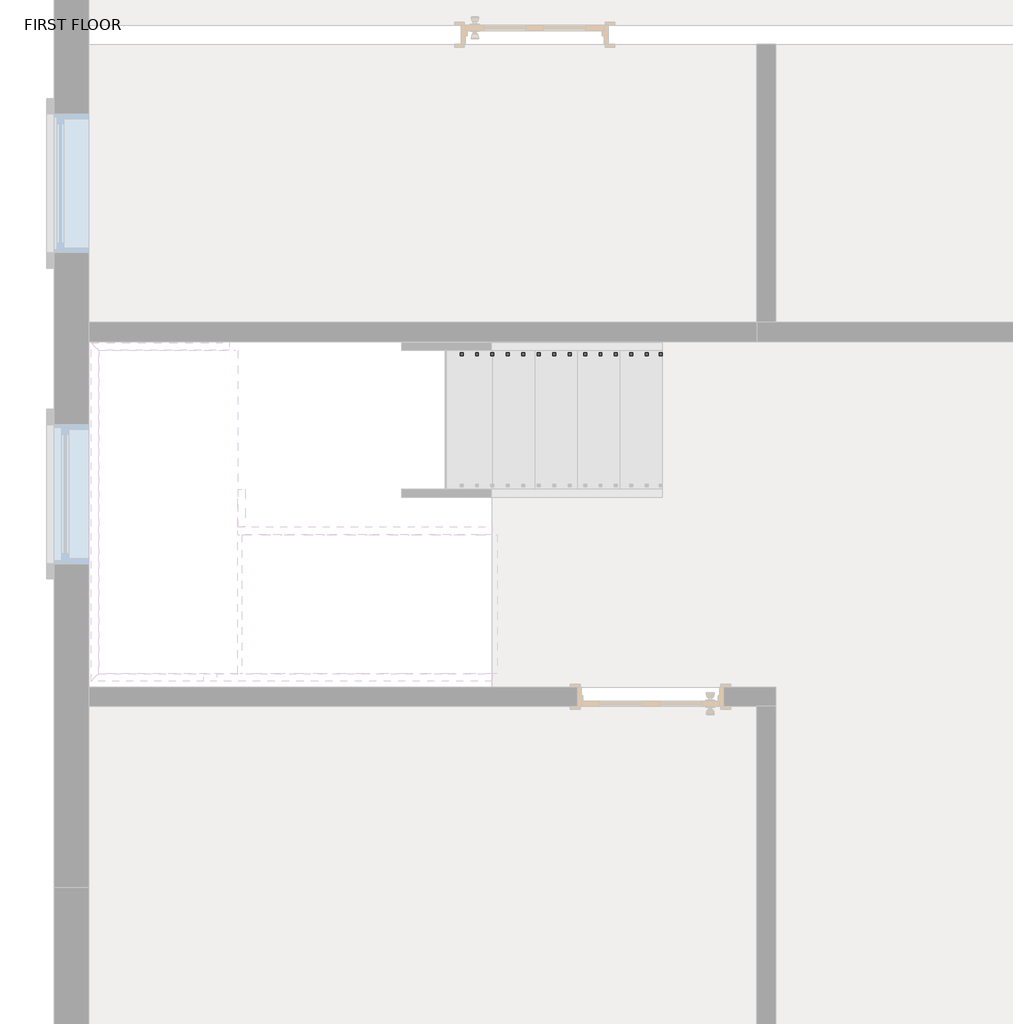
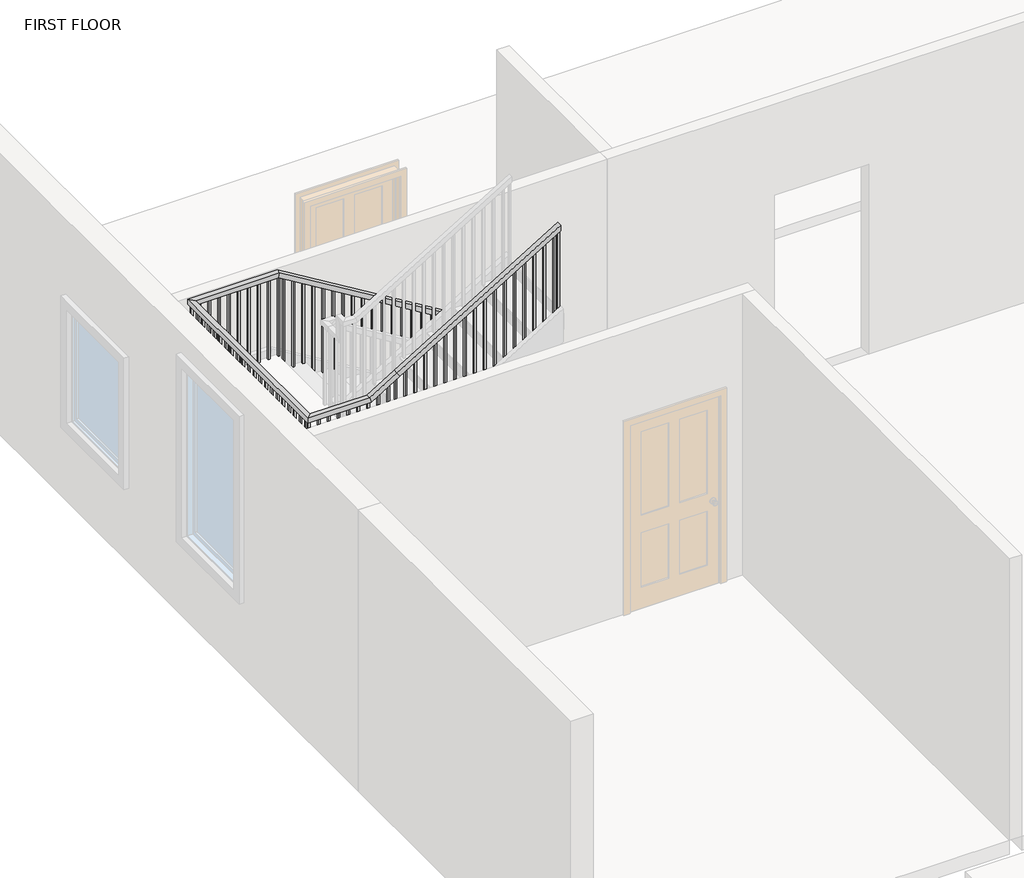
# One storey, part 3 of 4: 1 railing.
"""IFC4 building model written with IfcOpenShell, lengths in millimetres."""

from ifc_helpers import new_model, si_unit, frame, origin, place, context, project, spatial, polyline, outline, extrude, faceted_brep, element, save

model = new_model("IFC4")

# Units and contexts
model_context = context("Model", 3, world=origin())
ifc_project = project(units=[si_unit("LENGTHUNIT", "METRE", prefix="MILLI")], contexts=[model_context])

# Site, building, storey
site = spatial("IfcSite", under=ifc_project)
building = spatial("IfcBuilding", under=site)
storey = spatial("IfcBuildingStorey", under=building, Name="FIRST FLOOR", Elevation=3352.8)

# Railing
placement = place(None, origin())
element("IfcRailing", 1, ObjectType="Handrail - Rectangular", at=placement, inside=storey, context=model_context, shape_type="SolidModel", body=[
    faceted_brep([(-5990.8517085, 2868.2826226, 4741.3333333), (-5990.8517085, 2868.2826226, 4681.9318731), (-5990.8517085, 2919.0826226, 4681.9318731), (-5990.8517085, 2919.0826226, 4741.3333333), (-8784.8517085, 2868.2826226, 6434.6666667), (-8799.0441179, 2868.2826226, 6383.8666667), (-8799.0441179, 2919.0826226, 6383.8666667), (-8784.8517085, 2919.0826226, 6434.6666667), (-9648.4517085, 2868.2826226, 6434.6666667), (-9648.4517085, 2868.2826226, 6383.8666667), (-9699.2517085, 2919.0826226, 6383.8666667), (-9699.2517085, 2919.0826226, 6434.6666667), (-9648.4517085, 842.8165128, 6434.6666667), (-9648.4517085, 842.8165128, 6383.8666667), (-9699.2517085, 792.0165128, 6383.8666667), (-9699.2517085, 792.0165128, 6434.6666667), (-9064.2517085, 842.8165128, 6434.6666667), (-9050.0592991, 842.8165128, 6383.8666667), (-9050.0592991, 792.0165128, 6383.8666667), (-9064.2517085, 792.0165128, 6434.6666667), (-8784.8517085, 842.8165128, 6604.0), (-8758.5219813, 842.8165128, 6560.5559502), (-8758.5219813, 792.0165128, 6560.5559502), (-8784.8517085, 792.0165128, 6604.0), (-7108.4517085, 842.8165128, 7620.0), (-7108.4517085, 792.0165128, 7620.0), (-7108.4517085, 792.0165128, 7560.5985397), (-7108.4517085, 842.8165128, 7560.5985397)], [[[0, 1, 2, 3]], [[1, 0, 4, 5]], [[2, 1, 5, 6]], [[3, 2, 6, 7]], [[0, 3, 7, 4]], [[5, 4, 8, 9]], [[6, 5, 9, 10]], [[7, 6, 10, 11]], [[4, 7, 11, 8]], [[9, 8, 12, 13]], [[10, 9, 13, 14]], [[11, 10, 14, 15]], [[8, 11, 15, 12]], [[13, 12, 16, 17]], [[14, 13, 17, 18]], [[15, 14, 18, 19]], [[12, 15, 19, 16]], [[17, 16, 20, 21]], [[18, 17, 21, 22]], [[19, 18, 22, 23]], [[16, 19, 23, 20]], [[24, 25, 26, 27]], [[21, 20, 24, 27]], [[22, 21, 27, 26]], [[23, 22, 26, 25]], [[20, 23, 25, 24]]]),
    extrude(outline(polyline([(7535.5833882, -7149.7267085), (7524.0379337, -7168.7767085), (6536.2666667, -7168.7767085), (6536.2666667, -7149.7267085), (7535.5833882, -7149.7267085)])), frame((0.0, 807.8915128, 0.0), z_axis=(0.0, 1.0, 0.0), x_axis=(0.0, 0.0, 1.0)), (0.0, 0.0, 1.0), 19.05),
    extrude(outline(polyline([(7474.0076307, -7251.3267085), (7462.4621761, -7270.3767085), (6536.2666667, -7270.3767085), (6536.2666667, -7251.3267085), (7474.0076307, -7251.3267085)])), frame((0.0, 807.8915128, 0.0), z_axis=(0.0, 1.0, 0.0), x_axis=(0.0, 0.0, 1.0)), (0.0, 0.0, 1.0), 19.05),
    extrude(outline(polyline([(7412.4318731, -7352.9267085), (7400.8864185, -7371.9767085), (6536.2666667, -7371.9767085), (6536.2666667, -7352.9267085), (7412.4318731, -7352.9267085)])), frame((0.0, 807.8915128, 0.0), z_axis=(0.0, 1.0, 0.0), x_axis=(0.0, 0.0, 1.0)), (0.0, 0.0, 1.0), 19.05),
    extrude(outline(polyline([(7350.8561155, -7454.5267085), (7339.310661, -7473.5767085), (6366.9333333, -7473.5767085), (6366.9333333, -7454.5267085), (7350.8561155, -7454.5267085)])), frame((0.0, 807.8915128, 0.0), z_axis=(0.0, 1.0, 0.0), x_axis=(0.0, 0.0, 1.0)), (0.0, 0.0, 1.0), 19.05),
    extrude(outline(polyline([(7289.2803579, -7556.1267085), (7277.7349034, -7575.1767085), (6366.9333333, -7575.1767085), (6366.9333333, -7556.1267085), (7289.2803579, -7556.1267085)])), frame((0.0, 807.8915128, 0.0), z_axis=(0.0, 1.0, 0.0), x_axis=(0.0, 0.0, 1.0)), (0.0, 0.0, 1.0), 19.05),
    extrude(outline(polyline([(7227.7046004, -7657.7267085), (7216.1591458, -7676.7767085), (6366.9333333, -7676.7767085), (6366.9333333, -7657.7267085), (7227.7046004, -7657.7267085)])), frame((0.0, 807.8915128, 0.0), z_axis=(0.0, 1.0, 0.0), x_axis=(0.0, 0.0, 1.0)), (0.0, 0.0, 1.0), 19.05),
    extrude(outline(polyline([(7166.1288428, -7759.3267085), (7154.5833882, -7778.3767085), (6197.6, -7778.3767085), (6197.6, -7759.3267085), (7166.1288428, -7759.3267085)])), frame((0.0, 807.8915128, 0.0), z_axis=(0.0, 1.0, 0.0), x_axis=(0.0, 0.0, 1.0)), (0.0, 0.0, 1.0), 19.05),
    extrude(outline(polyline([(7104.5530852, -7860.9267085), (7093.0076307, -7879.9767085), (6197.6, -7879.9767085), (6197.6, -7860.9267085), (7104.5530852, -7860.9267085)])), frame((0.0, 807.8915128, 0.0), z_axis=(0.0, 1.0, 0.0), x_axis=(0.0, 0.0, 1.0)), (0.0, 0.0, 1.0), 19.05),
    extrude(outline(polyline([(7042.9773276, -7962.5267085), (7031.4318731, -7981.5767085), (6028.2666667, -7981.5767085), (6028.2666667, -7962.5267085), (7042.9773276, -7962.5267085)])), frame((0.0, 807.8915128, 0.0), z_axis=(0.0, 1.0, 0.0), x_axis=(0.0, 0.0, 1.0)), (0.0, 0.0, 1.0), 19.05),
    extrude(outline(polyline([(6981.40157, -8064.1267085), (6969.8561155, -8083.1767085), (6028.2666667, -8083.1767085), (6028.2666667, -8064.1267085), (6981.40157, -8064.1267085)])), frame((0.0, 807.8915128, 0.0), z_axis=(0.0, 1.0, 0.0), x_axis=(0.0, 0.0, 1.0)), (0.0, 0.0, 1.0), 19.05),
    extrude(outline(polyline([(6919.8258125, -8165.7267085), (6908.2803579, -8184.7767085), (6028.2666667, -8184.7767085), (6028.2666667, -8165.7267085), (6919.8258125, -8165.7267085)])), frame((0.0, 807.8915128, 0.0), z_axis=(0.0, 1.0, 0.0), x_axis=(0.0, 0.0, 1.0)), (0.0, 0.0, 1.0), 19.05),
    extrude(outline(polyline([(6858.2500549, -8267.3267085), (6846.7046004, -8286.3767085), (5858.9333333, -8286.3767085), (5858.9333333, -8267.3267085), (6858.2500549, -8267.3267085)])), frame((0.0, 807.8915128, 0.0), z_axis=(0.0, 1.0, 0.0), x_axis=(0.0, 0.0, 1.0)), (0.0, 0.0, 1.0), 19.05),
    extrude(outline(polyline([(6796.6742973, -8368.9267085), (6785.1288428, -8387.9767085), (5858.9333333, -8387.9767085), (5858.9333333, -8368.9267085), (6796.6742973, -8368.9267085)])), frame((0.0, 807.8915128, 0.0), z_axis=(0.0, 1.0, 0.0), x_axis=(0.0, 0.0, 1.0)), (0.0, 0.0, 1.0), 19.05),
    extrude(outline(polyline([(6735.0985397, -8470.5267085), (6723.5530852, -8489.5767085), (5858.9333333, -8489.5767085), (5858.9333333, -8470.5267085), (6735.0985397, -8470.5267085)])), frame((0.0, 807.8915128, 0.0), z_axis=(0.0, 1.0, 0.0), x_axis=(0.0, 0.0, 1.0)), (0.0, 0.0, 1.0), 19.05),
    extrude(outline(polyline([(6673.5227822, -8572.1267085), (6661.9773276, -8591.1767085), (5689.6, -8591.1767085), (5689.6, -8572.1267085), (6673.5227822, -8572.1267085)])), frame((0.0, 807.8915128, 0.0), z_axis=(0.0, 1.0, 0.0), x_axis=(0.0, 0.0, 1.0)), (0.0, 0.0, 1.0), 19.05),
    extrude(outline(polyline([(6611.9470246, -8673.7267085), (6600.40157, -8692.7767085), (5689.6, -8692.7767085), (5689.6, -8673.7267085), (6611.9470246, -8673.7267085)])), frame((0.0, 807.8915128, 0.0), z_axis=(0.0, 1.0, 0.0), x_axis=(0.0, 0.0, 1.0)), (0.0, 0.0, 1.0), 19.05),
    extrude(outline(polyline([(6504.1894488, -8851.5267085), (6492.6439943, -8870.5767085), (5520.2666667, -8870.5767085), (5520.2666667, -8851.5267085), (6504.1894488, -8851.5267085)])), frame((0.0, 807.8915128, 0.0), z_axis=(0.0, 1.0, 0.0), x_axis=(0.0, 0.0, 1.0)), (0.0, 0.0, 1.0), 19.05),
    extrude(outline(polyline([(6442.6136913, -8953.1267085), (6431.0682367, -8972.1767085), (5520.2666667, -8972.1767085), (5520.2666667, -8953.1267085), (6442.6136913, -8953.1267085)])), frame((0.0, 807.8915128, 0.0), z_axis=(0.0, 1.0, 0.0), x_axis=(0.0, 0.0, 1.0)), (0.0, 0.0, 1.0), 19.05),
    extrude(outline(polyline([(-9073.7767085, 807.8915128), (-9073.7767085, 826.9415128), (-9054.7267085, 826.9415128), (-9054.7267085, 807.8915128), (-9073.7767085, 807.8915128)])), frame((0.0, 0.0, 5520.2666667), z_axis=(0.0, 0.0, 1.0), x_axis=(1.0, 0.0, 0.0)), (0.0, 0.0, 1.0), 863.6),
    extrude(outline(polyline([(-9175.3767085, 807.8915128), (-9175.3767085, 826.9415128), (-9156.3267085, 826.9415128), (-9156.3267085, 807.8915128), (-9175.3767085, 807.8915128)])), frame((0.0, 0.0, 5520.2666667), z_axis=(0.0, 0.0, 1.0), x_axis=(1.0, 0.0, 0.0)), (0.0, 0.0, 1.0), 863.6),
    extrude(outline(polyline([(-9276.9767085, 807.8915128), (-9276.9767085, 826.9415128), (-9257.9267085, 826.9415128), (-9257.9267085, 807.8915128), (-9276.9767085, 807.8915128)])), frame((0.0, 0.0, 5520.2666667), z_axis=(0.0, 0.0, 1.0), x_axis=(1.0, 0.0, 0.0)), (0.0, 0.0, 1.0), 863.6),
    extrude(outline(polyline([(-9378.5767085, 807.8915128), (-9378.5767085, 826.9415128), (-9359.5267085, 826.9415128), (-9359.5267085, 807.8915128), (-9378.5767085, 807.8915128)])), frame((0.0, 0.0, 5520.2666667), z_axis=(0.0, 0.0, 1.0), x_axis=(1.0, 0.0, 0.0)), (0.0, 0.0, 1.0), 863.6),
    extrude(outline(polyline([(-9480.1767085, 807.8915128), (-9480.1767085, 826.9415128), (-9461.1267085, 826.9415128), (-9461.1267085, 807.8915128), (-9480.1767085, 807.8915128)])), frame((0.0, 0.0, 5520.2666667), z_axis=(0.0, 0.0, 1.0), x_axis=(1.0, 0.0, 0.0)), (0.0, 0.0, 1.0), 863.6),
    extrude(outline(polyline([(-9581.7767085, 807.8915128), (-9581.7767085, 826.9415128), (-9562.7267085, 826.9415128), (-9562.7267085, 807.8915128), (-9581.7767085, 807.8915128)])), frame((0.0, 0.0, 5520.2666667), z_axis=(0.0, 0.0, 1.0), x_axis=(1.0, 0.0, 0.0)), (0.0, 0.0, 1.0), 863.6),
    extrude(outline(polyline([(-9683.3767085, 871.2076226), (-9664.3267085, 871.2076226), (-9664.3267085, 852.1576226), (-9683.3767085, 852.1576226), (-9683.3767085, 871.2076226)])), frame((0.0, 0.0, 5520.2666667), z_axis=(0.0, 0.0, 1.0), x_axis=(1.0, 0.0, 0.0)), (0.0, 0.0, 1.0), 863.6),
    extrude(outline(polyline([(-9683.3767085, 972.8076226), (-9664.3267085, 972.8076226), (-9664.3267085, 953.7576226), (-9683.3767085, 953.7576226), (-9683.3767085, 972.8076226)])), frame((0.0, 0.0, 5520.2666667), z_axis=(0.0, 0.0, 1.0), x_axis=(1.0, 0.0, 0.0)), (0.0, 0.0, 1.0), 863.6),
    extrude(outline(polyline([(-9683.3767085, 1074.4076226), (-9664.3267085, 1074.4076226), (-9664.3267085, 1055.3576226), (-9683.3767085, 1055.3576226), (-9683.3767085, 1074.4076226)])), frame((0.0, 0.0, 5520.2666667), z_axis=(0.0, 0.0, 1.0), x_axis=(1.0, 0.0, 0.0)), (0.0, 0.0, 1.0), 863.6),
    extrude(outline(polyline([(-9683.3767085, 1176.0076226), (-9664.3267085, 1176.0076226), (-9664.3267085, 1156.9576226), (-9683.3767085, 1156.9576226), (-9683.3767085, 1176.0076226)])), frame((0.0, 0.0, 5520.2666667), z_axis=(0.0, 0.0, 1.0), x_axis=(1.0, 0.0, 0.0)), (0.0, 0.0, 1.0), 863.6),
    extrude(outline(polyline([(-9683.3767085, 1277.6076226), (-9664.3267085, 1277.6076226), (-9664.3267085, 1258.5576226), (-9683.3767085, 1258.5576226), (-9683.3767085, 1277.6076226)])), frame((0.0, 0.0, 5520.2666667), z_axis=(0.0, 0.0, 1.0), x_axis=(1.0, 0.0, 0.0)), (0.0, 0.0, 1.0), 863.6),
    extrude(outline(polyline([(-9683.3767085, 1379.2076226), (-9664.3267085, 1379.2076226), (-9664.3267085, 1360.1576226), (-9683.3767085, 1360.1576226), (-9683.3767085, 1379.2076226)])), frame((0.0, 0.0, 5520.2666667), z_axis=(0.0, 0.0, 1.0), x_axis=(1.0, 0.0, 0.0)), (0.0, 0.0, 1.0), 863.6),
    extrude(outline(polyline([(-9683.3767085, 1480.8076226), (-9664.3267085, 1480.8076226), (-9664.3267085, 1461.7576226), (-9683.3767085, 1461.7576226), (-9683.3767085, 1480.8076226)])), frame((0.0, 0.0, 5520.2666667), z_axis=(0.0, 0.0, 1.0), x_axis=(1.0, 0.0, 0.0)), (0.0, 0.0, 1.0), 863.6),
    extrude(outline(polyline([(-9683.3767085, 1582.4076226), (-9664.3267085, 1582.4076226), (-9664.3267085, 1563.3576226), (-9683.3767085, 1563.3576226), (-9683.3767085, 1582.4076226)])), frame((0.0, 0.0, 5520.2666667), z_axis=(0.0, 0.0, 1.0), x_axis=(1.0, 0.0, 0.0)), (0.0, 0.0, 1.0), 863.6),
    extrude(outline(polyline([(-9683.3767085, 1684.0076226), (-9664.3267085, 1684.0076226), (-9664.3267085, 1664.9576226), (-9683.3767085, 1664.9576226), (-9683.3767085, 1684.0076226)])), frame((0.0, 0.0, 5520.2666667), z_axis=(0.0, 0.0, 1.0), x_axis=(1.0, 0.0, 0.0)), (0.0, 0.0, 1.0), 863.6),
    extrude(outline(polyline([(-9683.3767085, 1785.6076226), (-9664.3267085, 1785.6076226), (-9664.3267085, 1766.5576226), (-9683.3767085, 1766.5576226), (-9683.3767085, 1785.6076226)])), frame((0.0, 0.0, 5520.2666667), z_axis=(0.0, 0.0, 1.0), x_axis=(1.0, 0.0, 0.0)), (0.0, 0.0, 1.0), 863.6),
    extrude(outline(polyline([(-9683.3767085, 1887.2076226), (-9664.3267085, 1887.2076226), (-9664.3267085, 1868.1576226), (-9683.3767085, 1868.1576226), (-9683.3767085, 1887.2076226)])), frame((0.0, 0.0, 5520.2666667), z_axis=(0.0, 0.0, 1.0), x_axis=(1.0, 0.0, 0.0)), (0.0, 0.0, 1.0), 863.6),
    extrude(outline(polyline([(-9683.3767085, 1988.8076226), (-9664.3267085, 1988.8076226), (-9664.3267085, 1969.7576226), (-9683.3767085, 1969.7576226), (-9683.3767085, 1988.8076226)])), frame((0.0, 0.0, 5520.2666667), z_axis=(0.0, 0.0, 1.0), x_axis=(1.0, 0.0, 0.0)), (0.0, 0.0, 1.0), 863.6),
    extrude(outline(polyline([(-9683.3767085, 2090.4076226), (-9664.3267085, 2090.4076226), (-9664.3267085, 2071.3576226), (-9683.3767085, 2071.3576226), (-9683.3767085, 2090.4076226)])), frame((0.0, 0.0, 5520.2666667), z_axis=(0.0, 0.0, 1.0), x_axis=(1.0, 0.0, 0.0)), (0.0, 0.0, 1.0), 863.6),
    extrude(outline(polyline([(-9683.3767085, 2192.0076226), (-9664.3267085, 2192.0076226), (-9664.3267085, 2172.9576226), (-9683.3767085, 2172.9576226), (-9683.3767085, 2192.0076226)])), frame((0.0, 0.0, 5520.2666667), z_axis=(0.0, 0.0, 1.0), x_axis=(1.0, 0.0, 0.0)), (0.0, 0.0, 1.0), 863.6),
    extrude(outline(polyline([(-9683.3767085, 2293.6076226), (-9664.3267085, 2293.6076226), (-9664.3267085, 2274.5576226), (-9683.3767085, 2274.5576226), (-9683.3767085, 2293.6076226)])), frame((0.0, 0.0, 5520.2666667), z_axis=(0.0, 0.0, 1.0), x_axis=(1.0, 0.0, 0.0)), (0.0, 0.0, 1.0), 863.6),
    extrude(outline(polyline([(-9683.3767085, 2395.2076226), (-9664.3267085, 2395.2076226), (-9664.3267085, 2376.1576226), (-9683.3767085, 2376.1576226), (-9683.3767085, 2395.2076226)])), frame((0.0, 0.0, 5520.2666667), z_axis=(0.0, 0.0, 1.0), x_axis=(1.0, 0.0, 0.0)), (0.0, 0.0, 1.0), 863.6),
    extrude(outline(polyline([(-9683.3767085, 2496.8076226), (-9664.3267085, 2496.8076226), (-9664.3267085, 2477.7576226), (-9683.3767085, 2477.7576226), (-9683.3767085, 2496.8076226)])), frame((0.0, 0.0, 5520.2666667), z_axis=(0.0, 0.0, 1.0), x_axis=(1.0, 0.0, 0.0)), (0.0, 0.0, 1.0), 863.6),
    extrude(outline(polyline([(-9683.3767085, 2598.4076226), (-9664.3267085, 2598.4076226), (-9664.3267085, 2579.3576226), (-9683.3767085, 2579.3576226), (-9683.3767085, 2598.4076226)])), frame((0.0, 0.0, 5520.2666667), z_axis=(0.0, 0.0, 1.0), x_axis=(1.0, 0.0, 0.0)), (0.0, 0.0, 1.0), 863.6),
    extrude(outline(polyline([(-9683.3767085, 2700.0076226), (-9664.3267085, 2700.0076226), (-9664.3267085, 2680.9576226), (-9683.3767085, 2680.9576226), (-9683.3767085, 2700.0076226)])), frame((0.0, 0.0, 5520.2666667), z_axis=(0.0, 0.0, 1.0), x_axis=(1.0, 0.0, 0.0)), (0.0, 0.0, 1.0), 863.6),
    extrude(outline(polyline([(-9683.3767085, 2801.6076226), (-9664.3267085, 2801.6076226), (-9664.3267085, 2782.5576226), (-9683.3767085, 2782.5576226), (-9683.3767085, 2801.6076226)])), frame((0.0, 0.0, 5520.2666667), z_axis=(0.0, 0.0, 1.0), x_axis=(1.0, 0.0, 0.0)), (0.0, 0.0, 1.0), 863.6),
    extrude(outline(polyline([(-9588.1267085, 2903.2076226), (-9588.1267085, 2884.1576226), (-9607.1767085, 2884.1576226), (-9607.1767085, 2903.2076226), (-9588.1267085, 2903.2076226)])), frame((0.0, 0.0, 5520.2666667), z_axis=(0.0, 0.0, 1.0), x_axis=(1.0, 0.0, 0.0)), (0.0, 0.0, 1.0), 863.6),
    extrude(outline(polyline([(-9486.5267085, 2903.2076226), (-9486.5267085, 2884.1576226), (-9505.5767085, 2884.1576226), (-9505.5767085, 2903.2076226), (-9486.5267085, 2903.2076226)])), frame((0.0, 0.0, 5520.2666667), z_axis=(0.0, 0.0, 1.0), x_axis=(1.0, 0.0, 0.0)), (0.0, 0.0, 1.0), 863.6),
    extrude(outline(polyline([(-9384.9267085, 2903.2076226), (-9384.9267085, 2884.1576226), (-9403.9767085, 2884.1576226), (-9403.9767085, 2903.2076226), (-9384.9267085, 2903.2076226)])), frame((0.0, 0.0, 5520.2666667), z_axis=(0.0, 0.0, 1.0), x_axis=(1.0, 0.0, 0.0)), (0.0, 0.0, 1.0), 863.6),
    extrude(outline(polyline([(-9283.3267085, 2903.2076226), (-9283.3267085, 2884.1576226), (-9302.3767085, 2884.1576226), (-9302.3767085, 2903.2076226), (-9283.3267085, 2903.2076226)])), frame((0.0, 0.0, 5520.2666667), z_axis=(0.0, 0.0, 1.0), x_axis=(1.0, 0.0, 0.0)), (0.0, 0.0, 1.0), 863.6),
    extrude(outline(polyline([(-9181.7267085, 2903.2076226), (-9181.7267085, 2884.1576226), (-9200.7767085, 2884.1576226), (-9200.7767085, 2903.2076226), (-9181.7267085, 2903.2076226)])), frame((0.0, 0.0, 5520.2666667), z_axis=(0.0, 0.0, 1.0), x_axis=(1.0, 0.0, 0.0)), (0.0, 0.0, 1.0), 863.6),
    extrude(outline(polyline([(-9080.1267085, 2903.2076226), (-9080.1267085, 2884.1576226), (-9099.1767085, 2884.1576226), (-9099.1767085, 2903.2076226), (-9080.1267085, 2903.2076226)])), frame((0.0, 0.0, 5520.2666667), z_axis=(0.0, 0.0, 1.0), x_axis=(1.0, 0.0, 0.0)), (0.0, 0.0, 1.0), 863.6),
    extrude(outline(polyline([(-8978.5267085, 2903.2076226), (-8978.5267085, 2884.1576226), (-8997.5767085, 2884.1576226), (-8997.5767085, 2903.2076226), (-8978.5267085, 2903.2076226)])), frame((0.0, 0.0, 5520.2666667), z_axis=(0.0, 0.0, 1.0), x_axis=(1.0, 0.0, 0.0)), (0.0, 0.0, 1.0), 863.6),
    extrude(outline(polyline([(-8876.9267085, 2903.2076226), (-8876.9267085, 2884.1576226), (-8895.9767085, 2884.1576226), (-8895.9767085, 2903.2076226), (-8876.9267085, 2903.2076226)])), frame((0.0, 0.0, 5520.2666667), z_axis=(0.0, 0.0, 1.0), x_axis=(1.0, 0.0, 0.0)), (0.0, 0.0, 1.0), 863.6),
    extrude(outline(polyline([(6338.7046004, -8724.5267085), (6350.2500549, -8743.5767085), (5350.9333333, -8743.5767085), (5350.9333333, -8724.5267085), (6338.7046004, -8724.5267085)])), frame((0.0, 2884.1576226, 0.0), z_axis=(0.0, 1.0, 0.0), x_axis=(0.0, 0.0, 1.0)), (0.0, 0.0, 1.0), 19.05),
    extrude(outline(polyline([(6277.1288428, -8622.9267085), (6288.6742973, -8641.9767085), (5350.9333333, -8641.9767085), (5350.9333333, -8622.9267085), (6277.1288428, -8622.9267085)])), frame((0.0, 2884.1576226, 0.0), z_axis=(0.0, 1.0, 0.0), x_axis=(0.0, 0.0, 1.0)), (0.0, 0.0, 1.0), 19.05),
    extrude(outline(polyline([(6215.5530852, -8521.3267085), (6227.0985397, -8540.3767085), (5350.9333333, -8540.3767085), (5350.9333333, -8521.3267085), (6215.5530852, -8521.3267085)])), frame((0.0, 2884.1576226, 0.0), z_axis=(0.0, 1.0, 0.0), x_axis=(0.0, 0.0, 1.0)), (0.0, 0.0, 1.0), 19.05),
    extrude(outline(polyline([(6153.9773276, -8419.7267085), (6165.5227822, -8438.7767085), (5181.6, -8438.7767085), (5181.6, -8419.7267085), (6153.9773276, -8419.7267085)])), frame((0.0, 2884.1576226, 0.0), z_axis=(0.0, 1.0, 0.0), x_axis=(0.0, 0.0, 1.0)), (0.0, 0.0, 1.0), 19.05),
    extrude(outline(polyline([(6092.40157, -8318.1267085), (6103.9470246, -8337.1767085), (5181.6, -8337.1767085), (5181.6, -8318.1267085), (6092.40157, -8318.1267085)])), frame((0.0, 2884.1576226, 0.0), z_axis=(0.0, 1.0, 0.0), x_axis=(0.0, 0.0, 1.0)), (0.0, 0.0, 1.0), 19.05),
    extrude(outline(polyline([(6030.8258125, -8216.5267085), (6042.371267, -8235.5767085), (5181.6, -8235.5767085), (5181.6, -8216.5267085), (6030.8258125, -8216.5267085)])), frame((0.0, 2884.1576226, 0.0), z_axis=(0.0, 1.0, 0.0), x_axis=(0.0, 0.0, 1.0)), (0.0, 0.0, 1.0), 19.05),
    extrude(outline(polyline([(5969.2500549, -8114.9267085), (5980.7955094, -8133.9767085), (5012.2666667, -8133.9767085), (5012.2666667, -8114.9267085), (5969.2500549, -8114.9267085)])), frame((0.0, 2884.1576226, 0.0), z_axis=(0.0, 1.0, 0.0), x_axis=(0.0, 0.0, 1.0)), (0.0, 0.0, 1.0), 19.05),
    extrude(outline(polyline([(5907.6742973, -8013.3267085), (5919.2197519, -8032.3767085), (5012.2666667, -8032.3767085), (5012.2666667, -8013.3267085), (5907.6742973, -8013.3267085)])), frame((0.0, 2884.1576226, 0.0), z_axis=(0.0, 1.0, 0.0), x_axis=(0.0, 0.0, 1.0)), (0.0, 0.0, 1.0), 19.05),
    extrude(outline(polyline([(5846.0985397, -7911.7267085), (5857.6439943, -7930.7767085), (4842.9333333, -7930.7767085), (4842.9333333, -7911.7267085), (5846.0985397, -7911.7267085)])), frame((0.0, 2884.1576226, 0.0), z_axis=(0.0, 1.0, 0.0), x_axis=(0.0, 0.0, 1.0)), (0.0, 0.0, 1.0), 19.05),
    extrude(outline(polyline([(5784.5227822, -7810.1267085), (5796.0682367, -7829.1767085), (4842.9333333, -7829.1767085), (4842.9333333, -7810.1267085), (5784.5227822, -7810.1267085)])), frame((0.0, 2884.1576226, 0.0), z_axis=(0.0, 1.0, 0.0), x_axis=(0.0, 0.0, 1.0)), (0.0, 0.0, 1.0), 19.05),
    extrude(outline(polyline([(5722.9470246, -7708.5267085), (5734.4924791, -7727.5767085), (4842.9333333, -7727.5767085), (4842.9333333, -7708.5267085), (5722.9470246, -7708.5267085)])), frame((0.0, 2884.1576226, 0.0), z_axis=(0.0, 1.0, 0.0), x_axis=(0.0, 0.0, 1.0)), (0.0, 0.0, 1.0), 19.05),
    extrude(outline(polyline([(5661.371267, -7606.9267085), (5672.9167216, -7625.9767085), (4673.6, -7625.9767085), (4673.6, -7606.9267085), (5661.371267, -7606.9267085)])), frame((0.0, 2884.1576226, 0.0), z_axis=(0.0, 1.0, 0.0), x_axis=(0.0, 0.0, 1.0)), (0.0, 0.0, 1.0), 19.05),
    extrude(outline(polyline([(5599.7955094, -7505.3267085), (5611.340964, -7524.3767085), (4673.6, -7524.3767085), (4673.6, -7505.3267085), (5599.7955094, -7505.3267085)])), frame((0.0, 2884.1576226, 0.0), z_axis=(0.0, 1.0, 0.0), x_axis=(0.0, 0.0, 1.0)), (0.0, 0.0, 1.0), 19.05),
    extrude(outline(polyline([(5538.2197519, -7403.7267085), (5549.7652064, -7422.7767085), (4673.6, -7422.7767085), (4673.6, -7403.7267085), (5538.2197519, -7403.7267085)])), frame((0.0, 2884.1576226, 0.0), z_axis=(0.0, 1.0, 0.0), x_axis=(0.0, 0.0, 1.0)), (0.0, 0.0, 1.0), 19.05),
    extrude(outline(polyline([(5476.6439943, -7302.1267085), (5488.1894488, -7321.1767085), (4504.2666667, -7321.1767085), (4504.2666667, -7302.1267085), (5476.6439943, -7302.1267085)])), frame((0.0, 2884.1576226, 0.0), z_axis=(0.0, 1.0, 0.0), x_axis=(0.0, 0.0, 1.0)), (0.0, 0.0, 1.0), 19.05),
    extrude(outline(polyline([(5415.0682367, -7200.5267085), (5426.6136913, -7219.5767085), (4504.2666667, -7219.5767085), (4504.2666667, -7200.5267085), (5415.0682367, -7200.5267085)])), frame((0.0, 2884.1576226, 0.0), z_axis=(0.0, 1.0, 0.0), x_axis=(0.0, 0.0, 1.0)), (0.0, 0.0, 1.0), 19.05),
    extrude(outline(polyline([(5353.4924791, -7098.9267085), (5365.0379337, -7117.9767085), (4504.2666667, -7117.9767085), (4504.2666667, -7098.9267085), (5353.4924791, -7098.9267085)])), frame((0.0, 2884.1576226, 0.0), z_axis=(0.0, 1.0, 0.0), x_axis=(0.0, 0.0, 1.0)), (0.0, 0.0, 1.0), 19.05),
    extrude(outline(polyline([(5291.9167216, -6997.3267085), (5303.4621761, -7016.3767085), (4334.9333333, -7016.3767085), (4334.9333333, -6997.3267085), (5291.9167216, -6997.3267085)])), frame((0.0, 2884.1576226, 0.0), z_axis=(0.0, 1.0, 0.0), x_axis=(0.0, 0.0, 1.0)), (0.0, 0.0, 1.0), 19.05),
    extrude(outline(polyline([(5230.340964, -6895.7267085), (5241.8864185, -6914.7767085), (4334.9333333, -6914.7767085), (4334.9333333, -6895.7267085), (5230.340964, -6895.7267085)])), frame((0.0, 2884.1576226, 0.0), z_axis=(0.0, 1.0, 0.0), x_axis=(0.0, 0.0, 1.0)), (0.0, 0.0, 1.0), 19.05),
    extrude(outline(polyline([(5168.7652064, -6794.1267085), (5180.310661, -6813.1767085), (4165.6, -6813.1767085), (4165.6, -6794.1267085), (5168.7652064, -6794.1267085)])), frame((0.0, 2884.1576226, 0.0), z_axis=(0.0, 1.0, 0.0), x_axis=(0.0, 0.0, 1.0)), (0.0, 0.0, 1.0), 19.05),
    extrude(outline(polyline([(5107.1894488, -6692.5267085), (5118.7349034, -6711.5767085), (4165.6, -6711.5767085), (4165.6, -6692.5267085), (5107.1894488, -6692.5267085)])), frame((0.0, 2884.1576226, 0.0), z_axis=(0.0, 1.0, 0.0), x_axis=(0.0, 0.0, 1.0)), (0.0, 0.0, 1.0), 19.05),
    extrude(outline(polyline([(5045.6136913, -6590.9267085), (5057.1591458, -6609.9767085), (4165.6, -6609.9767085), (4165.6, -6590.9267085), (5045.6136913, -6590.9267085)])), frame((0.0, 2884.1576226, 0.0), z_axis=(0.0, 1.0, 0.0), x_axis=(0.0, 0.0, 1.0)), (0.0, 0.0, 1.0), 19.05),
    extrude(outline(polyline([(4984.0379337, -6489.3267085), (4995.5833882, -6508.3767085), (3996.2666667, -6508.3767085), (3996.2666667, -6489.3267085), (4984.0379337, -6489.3267085)])), frame((0.0, 2884.1576226, 0.0), z_axis=(0.0, 1.0, 0.0), x_axis=(0.0, 0.0, 1.0)), (0.0, 0.0, 1.0), 19.05),
    extrude(outline(polyline([(4922.4621761, -6387.7267085), (4934.0076307, -6406.7767085), (3996.2666667, -6406.7767085), (3996.2666667, -6387.7267085), (4922.4621761, -6387.7267085)])), frame((0.0, 2884.1576226, 0.0), z_axis=(0.0, 1.0, 0.0), x_axis=(0.0, 0.0, 1.0)), (0.0, 0.0, 1.0), 19.05),
    extrude(outline(polyline([(4860.8864185, -6286.1267085), (4872.4318731, -6305.1767085), (3996.2666667, -6305.1767085), (3996.2666667, -6286.1267085), (4860.8864185, -6286.1267085)])), frame((0.0, 2884.1576226, 0.0), z_axis=(0.0, 1.0, 0.0), x_axis=(0.0, 0.0, 1.0)), (0.0, 0.0, 1.0), 19.05),
    extrude(outline(polyline([(4799.310661, -6184.5267085), (4810.8561155, -6203.5767085), (3826.9333333, -6203.5767085), (3826.9333333, -6184.5267085), (4799.310661, -6184.5267085)])), frame((0.0, 2884.1576226, 0.0), z_axis=(0.0, 1.0, 0.0), x_axis=(0.0, 0.0, 1.0)), (0.0, 0.0, 1.0), 19.05),
    extrude(outline(polyline([(4737.7349034, -6082.9267085), (4749.2803579, -6101.9767085), (3826.9333333, -6101.9767085), (3826.9333333, -6082.9267085), (4737.7349034, -6082.9267085)])), frame((0.0, 2884.1576226, 0.0), z_axis=(0.0, 1.0, 0.0), x_axis=(0.0, 0.0, 1.0)), (0.0, 0.0, 1.0), 19.05),
    extrude(outline(polyline([(6550.371267, -8775.3267085), (6538.8258125, -8794.3767085), (5520.2666667, -8794.3767085), (5520.2666667, -8775.3267085), (6550.371267, -8775.3267085)])), frame((0.0, 807.8915128, 0.0), z_axis=(0.0, 1.0, 0.0), x_axis=(0.0, 0.0, 1.0)), (0.0, 0.0, 1.0), 19.05),
    extrude(outline(polyline([(-9683.3767085, 826.9415128), (-9664.3267085, 826.9415128), (-9664.3267085, 807.8915128), (-9683.3767085, 807.8915128), (-9683.3767085, 826.9415128)])), frame((0.0, 0.0, 5520.2666667), z_axis=(0.0, 0.0, 1.0), x_axis=(1.0, 0.0, 0.0)), (0.0, 0.0, 1.0), 863.6),
    extrude(outline(polyline([(-9664.3267085, 2903.2076226), (-9664.3267085, 2884.1576226), (-9683.3767085, 2884.1576226), (-9683.3767085, 2903.2076226), (-9664.3267085, 2903.2076226)])), frame((0.0, 0.0, 5520.2666667), z_axis=(0.0, 0.0, 1.0), x_axis=(1.0, 0.0, 0.0)), (0.0, 0.0, 1.0), 863.6),
    extrude(outline(polyline([(6369.4924791, -8775.3267085), (6381.0379337, -8794.3767085), (5520.2666667, -8794.3767085), (5520.2666667, -8775.3267085), (6369.4924791, -8775.3267085)])), frame((0.0, 2884.1576226, 0.0), z_axis=(0.0, 1.0, 0.0), x_axis=(0.0, 0.0, 1.0)), (0.0, 0.0, 1.0), 19.05),
    extrude(outline(polyline([(7560.5985397, -7108.4517085), (7549.0530852, -7127.5017085), (6536.2666667, -7127.5017085), (6536.2666667, -7108.4517085), (7560.5985397, -7108.4517085)])), frame((0.0, 807.8915128, 0.0), z_axis=(0.0, 1.0, 0.0), x_axis=(0.0, 0.0, 1.0)), (0.0, 0.0, 1.0), 19.05),
    extrude(outline(polyline([(4681.9318731, -5990.8517085), (4693.4773276, -6009.9017085), (3826.9333333, -6009.9017085), (3826.9333333, -5990.8517085), (4681.9318731, -5990.8517085)])), frame((0.0, 2884.1576226, 0.0), z_axis=(0.0, 1.0, 0.0), x_axis=(0.0, 0.0, 1.0)), (0.0, 0.0, 1.0), 19.05),
])

save(model, "model.ifc")

# Revit data of these elements
# Type "Handrail - Rectangular"
#   Assembly Code = "C2010400"
#   built-in parameter 1008612 = 0.0416667 (stored number, unit not read)
#   built-in parameter 1008611 = 0.0416667 (stored number, unit not read)
#   built-in parameter 1008609 = 0.333333 (stored number, unit not read)
#   built-in parameter 1008604 = 0.166667 (stored number, unit not read)
#   built-in parameter 1008603 = 0.166667 (stored number, unit not read)
#   Railing Height = 3' - 0"
#   built-in parameter 1008630 = 2
#   built-in parameter 1008610 = 2
#   built-in parameter 1008618 = Baluster - Square : 3/4"
# Element 1 (IfcRailing, "Handrail - Rectangular")
#   Phase Created = New Construction
